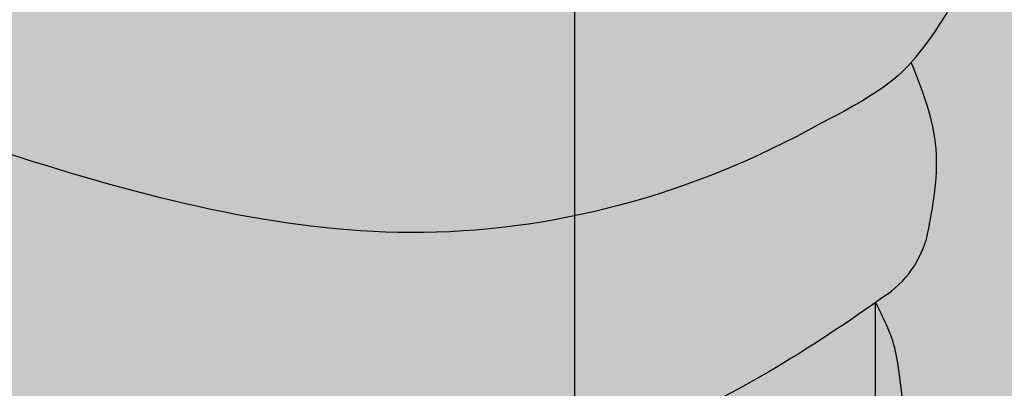
# Model space of a CAD drawing. Units: inches. Extents: x 1704 to 6393, y -157 to 1172.
# Tile 36 of 122: x 2526 to 2564, y 148 to 162. Entities that reach past the tile are written whole.
import ezdxf

# ---------------------------------------------------------------- set-up
doc = ezdxf.new("R2010")
doc.units = ezdxf.units.IN
doc.header["$MEASUREMENT"] = 0
for name, color, linetype, lineweight in [('A-ANNO-DIMS', 7, 'Continuous', 13), ('A-FURN', 8, 'Continuous', 18), ('estofado', 7, 'Continuous', 25)]:
    doc.layers.add(name, color=color, linetype=linetype, lineweight=lineweight)
doc.layers.add('A-FLOR-PATT', color=7, linetype='Continuous', lineweight=13, true_color=0xf2f2f2)
doc.styles.get("Standard").update_dxf_attribs({"font": 'arial.ttf'})
doc.dimstyles.get("Standard").update_dxf_attribs({"dimtxt": 6, "dimasz": 2, "dimexe": 0.18, "dimexo": 0.0625, "dimgap": 0.09, "dimtad": 0, "dimtih": 1, "dimtoh": 1, "dimdec": 1, "dimzin": 0, "dimdsep": 46, "dimlunit": 3, "dimtxsty": 'Standard', "dimblk": 'ARCHTICK', "dimcen": 0.09, "dimadec": 0, "dimazin": 0, "dimtfac": 1, "dimtdec": 1, "dimtofl": 0, "dimtmove": 0, "dimatfit": 3, "dimfxl": 1, "dimtolj": 1, "dimtzin": 0, "dimarcsym": 0})

# ---------------------------------------------------------------- blocks, each defined once
blk = doc.blocks.new('Cama Box Regencia LOLA')
at = {"layer": 'estofado', "ltscale": 0.2}
h = blk.add_hatch(color=256, dxfattribs=at)
h.dxf.hatch_style = 1
h.set_gradient(color1=(240, 232, 219), color2=(213, 190, 154), one_color=1, tint=0.7200000286102295)
edge = h.paths.add_edge_path()
edge.add_line((-0.8000000000000682, -0.1548023628405417), (-0.863597199697665, -0.2293271111754507))
edge.add_spline(control_points=[(-0.8635971996977787, -0.2293271111754507), (-0.8537222782123308, -0.258285373872468), (-0.8269013755602826, -0.3369378214810581), (-0.8674912876567759, -0.4595932758330151), (-0.8253488717912205, -0.6001498518888299), (-0.8771423076391329, -0.7139760714239288), (-0.8243323781925938, -0.8129899320257435), (-0.885044987287756, -0.8716602542656914), (-0.879518062107536, -0.9542863467743244), (-0.8339551707063037, -1.008464155856984), (-0.8245672924600739, -1.059984630119799), (-0.8208601923470268, -1.104655887174089), (-0.8073908324747662, -1.131238421004809), (-0.7999999999999546, -1.145824641594799)], knot_values=[0, 0, 0, 0, 0.0901802310564388, 0.2449351320798513, 0.3646438241986237, 0.5132330690395209, 0.5950634960661151, 0.646820388242338, 0.740988272125753, 0.8098674202588053, 0.8551784313864677, 0.8950360916221496, 0.9434986994854018, 0.9434986994854018, 0.9434986994854018, 0.9434986994854018], degree=3, periodic=0)
edge.add_line((-0.7999999999999546, -1.145824641594856), (-0.7999999999999546, -0.9571831923306604))
edge.add_spline(control_points=[(-0.8000000000001818, -0.9571831923294098), (-0.8003674620557603, -0.9560020588672273), (-0.8014778173377408, -0.9524330433489467), (-0.799534669348418, -0.9460450666617248), (-0.7963405736333016, -0.9382358308520792), (-0.7944188048602429, -0.9289040147384638), (-0.7953122817383474, -0.9190683391483389), (-0.7985341887020923, -0.9137677522519994), (-0.7999999999999546, -0.911356242470788)], knot_values=[0, 0, 0, 0, 0.0036609130031785, 0.0110621328900358, 0.0190316076023675, 0.0292873612819121, 0.0393286152452009, 0.0477100398955968, 0.0477100398955968, 0.0477100398955968, 0.0477100398955968], degree=3, periodic=0)
edge.add_line((-0.8000000000000682, -0.9113562424705037), (-0.7999999999999546, -0.8573491405791173))
edge.add_spline(control_points=[(-0.7999999999999546, -0.8573491405791173), (-0.8011509914009592, -0.8570771933481751), (-0.804102924754261, -0.8563797336621519), (-0.8039036519178353, -0.8498286502876908), (-0.8010279369466388, -0.8413595542568258), (-0.805623441450507, -0.8302818657685406), (-0.801318481758244, -0.8238273834048186), (-0.7999999999999546, -0.8218505664625013)], knot_values=[0, 0, 0, 0, 0.0032305881034183, 0.0082854491905874, 0.015951437769388, 0.0315866871777379, 0.0384893971878813, 0.0384893971878813, 0.0384893971878813, 0.0384893971878813], degree=3, periodic=0)
edge.add_line((-0.7999999999999546, -0.821850566462558), (-0.7999999999999546, -0.7800193173444541))
edge.add_spline(control_points=[(-0.7999999999999546, -0.7800193173443404), (-0.7985416092056994, -0.7788853679199974), (-0.7956241855360986, -0.7766169698310819), (-0.7929439183725436, -0.7707329795046576), (-0.7969680334608711, -0.7644035258254576), (-0.7912681985083055, -0.7566015403456845), (-0.7963938877088595, -0.7483952775559715), (-0.798936373489596, -0.7431699116222604), (-0.799999999999841, -0.7409839258539251)], knot_values=[0, 0, 0, 0, 0.0055481279082489, 0.0110986984731684, 0.0174746050947868, 0.0251556172852474, 0.035519246289823, 0.0429729849735991, 0.0429729849735991, 0.0429729849735991, 0.0429729849735991], degree=3, periodic=0)
edge.add_line((-0.7999999999999546, -0.740983925853584), (-0.8000000000000682, -0.1548023628405417))
h = blk.add_hatch(color=256, dxfattribs=at)
h.dxf.hatch_style = 1
h.set_gradient(color1=(240, 232, 219), color2=(213, 190, 154), one_color=1, tint=0.7200000286102295, name='CURVED')
edge = h.paths.add_edge_path()
edge.add_spline(control_points=[(0.343533776195045, -0.8455058148597345), (0.2879313990920309, -0.8167160606696484), (0.2054770794474052, -0.7744470032542381), (0.0954193394759386, -0.7742416952675626), (-0.0885363502328574, -0.7276964167006668), (0.2428192566063672, -0.7672518992321216), (0.345087521536243, -0.8076697826234067), (0.3825206986321063, -0.8228555492498799)], knot_values=[0.0056315103357428, 0.0056315103357428, 0.0056315103357428, 0.0056315103357428, 0.1860138916206105, 0.2660015162584448, 0.3570871810327863, 0.5963901805690979, 0.739731738908988, 0.739731738908988, 0.739731738908988, 0.739731738908988], degree=3, periodic=0)
edge.add_spline(control_points=[(0.3825206986325611, -0.8228555492497662), (0.3974221570828149, -0.8135511441712424), (0.4121061736600496, -0.8037181558521524), (0.4266849906532571, -0.7937075488799225)], knot_values=[1.358237767273279, 1.358237767273279, 1.358237767273279, 1.358237767273279, 1.409915662372559, 1.409915662372559, 1.409915662372559, 1.409915662372559], degree=3, periodic=0)
edge.add_spline(control_points=[(0.4266849905698109, -0.7937075489369932), (0.3998777739682282, -0.7821381809783361), (0.3476761897024971, -0.7634757898491671), (0.2670618099601825, -0.7565375622627358), (0.0835725072796549, -0.7192994417154637), (0.288524529784695, -0.7446405493717521), (0.4247448861246994, -0.7759943071475277), (0.4449816270193879, -0.7810438091316882)], knot_values=[0.1043639306803623, 0.1043639306803623, 0.1043639306803623, 0.1043639306803623, 0.1896363068641149, 0.2696239315019491, 0.3607095962762907, 0.6000125958126024, 0.6446217338078729, 0.6446217338078729, 0.6446217338078729, 0.6446217338078729], degree=3, periodic=0)
edge.add_spline(control_points=[(0.4449816270197289, -0.7810438091316882), (0.5029779388527232, -0.7406836481117695), (0.5966687145296419, -0.6736247633211292), (0.7071737530245628, -0.6656573253703187), (0.7517012483331201, -0.6672238302253392)], knot_values=[1.43159032281798, 1.43159032281798, 1.43159032281798, 1.43159032281798, 1.63814180148235, 1.770695287284994, 1.770695287284994, 1.770695287284994, 1.770695287284994], degree=3, periodic=0)
edge.add_arc((0.7481853615017826, -0.767162003811734), 0.0999999999999888, 58.7920033978138, 87.98512997550938, ccw=False)
edge.add_line((0.8000000000000682, -0.6816328085782289), (0.8000000000000682, -0.154802362840428))
edge.add_line((0.8000000000000682, -0.154802362840428), (-0.7999999999999546, -0.154802362840428))
edge.add_line((-0.7999999999999546, -0.154802362840428), (-0.8000000000000682, -0.7409839258539819))
edge.add_spline(control_points=[(-0.799999999999841, -0.7409839258539251), (-0.7846451382113174, -0.74846387981205), (-0.7568940913494089, -0.7651582159765554), (-0.7559936909002545, -0.8096905380045313), (-0.7049413305308008, -0.8142555457367848), (-0.7013836936888538, -0.8139988647640733)], knot_values=[0.0122267587020837, 0.0122267587020837, 0.0122267587020837, 0.0122267587020837, 0.0594720782072034, 0.1062176618094138, 0.134458043575382, 0.134458043575382, 0.134458043575382, 0.134458043575382], degree=3, periodic=0)
edge.add_spline(control_points=[(-0.7013836936890812, -0.8139988647637892), (-0.6428309483887916, -0.8132695376718857), (-0.532520673001045, -0.8118955240036598), (-0.2390712668254764, -0.6717984706609172), (-0.3892411364554391, -0.7557901092520752), (-0.4591093260188473, -0.8070101468627512), (-0.5571511178645779, -0.795652750469742), (-0.608497950975675, -0.8409486634728295), (-0.6632498050151981, -0.8266781836207997), (-0.6991149398675134, -0.8254126024436914), (-0.719552182989446, -0.8246914287938125)], knot_values=[0, 0, 0, 0, 0.2187005959148062, 0.4120203559900679, 0.4786136596093368, 0.6046444033330721, 0.6969970394608519, 0.7456449795902803, 0.7925683322559657, 0.8547274388453192, 0.8547274388453192, 0.8547274388453192, 0.8547274388453192], degree=3, periodic=0)
edge.add_spline(control_points=[(-0.7195521829781911, -0.824691428792164), (-0.7293124663336812, -0.8248308281530967), (-0.7545977292818407, -0.8216412233076653), (-0.7742556984202338, -0.794819860189591), (-0.7939222919129634, -0.7820064600295497), (-0.799999999999841, -0.7800193173443404)], knot_values=[0.1564883932805935, 0.1564883932805935, 0.1564883932805935, 0.1564883932805935, 0.184397548386913, 0.2313764834161266, 0.2505984550882281, 0.2505984550882281, 0.2505984550882281, 0.2505984550882281], degree=3, periodic=0)
edge.add_line((-0.8000000000000682, -0.7800193173444541), (-0.7999999999999546, -0.8218505664627286))
edge.add_spline(control_points=[(-0.7999999999999546, -0.8218505664625013), (-0.7938082505512511, -0.8290217081292894), (-0.7673857405620766, -0.8512914803976059), (-0.7619109683460011, -0.8661369353891359), (-0.6555700939965164, -0.8510070218793543), (-0.7139793977868294, -0.8637526923380391), (-0.7379026254519659, -0.8623504601624176), (-0.7688129786438367, -0.8813042143888196), (-0.7854260296310259, -0.8561610219318254), (-0.7961930533253962, -0.8566031243811949), (-0.7999999999999546, -0.8573491405791173)], knot_values=[0.0595743221876141, 0.0595743221876141, 0.0595743221876141, 0.0595743221876141, 0.08075289116965, 0.1037414994169835, 0.1697200936249022, 0.1760361327243865, 0.2071371586311508, 0.2404744334261798, 0.2623408547027293, 0.2736604507987723, 0.2736604507987723, 0.2736604507987723, 0.2736604507987723], degree=3, periodic=0)
edge.add_line((-0.7999999999999546, -0.8573491405791173), (-0.8000000000000682, -0.9113562424721521))
edge.add_spline(control_points=[(-0.8000000000000682, -0.9113562424720385), (-0.7937204054647964, -0.9077594990848183), (-0.7710343135782978, -0.8978798065321029), (-0.7213062468074442, -0.9144666877443228), (-0.6268586829058905, -0.862430497409548), (-0.6896594748232019, -0.9045634991654196), (-0.7483442493064559, -0.9189273406958591), (-0.7835301183422417, -0.922920432793262), (-0.7896301351460125, -0.9477657000142585), (-0.7975786973822779, -0.955260590410262), (-0.8000000000001818, -0.9571831923294098)], knot_values=[0.0138560263374175, 0.0138560263374175, 0.0138560263374175, 0.0138560263374175, 0.0348737775836104, 0.0888666909546002, 0.1078792274429341, 0.1267378491223226, 0.1587140219647659, 0.1937574699451985, 0.2174867851300671, 0.2267221218327879, 0.2267221218327879, 0.2267221218327879, 0.2267221218327879], degree=3, periodic=0)
edge.add_line((-0.7999999999999546, -0.957183192329296), (-0.7999999999999546, -1.145824641594742))
edge.add_spline(control_points=[(-0.8000000000002955, -1.145824641594913), (-0.7271039467997298, -1.094596787649038), (-0.4885706936571524, -0.9465888221489535), (-0.0701640902225336, -0.9707493165000187), (0.237911901821235, -0.902164522332157), (0.3435337762145991, -0.845505814843193)], knot_values=[0.1168958193629841, 0.1168958193629841, 0.1168958193629841, 0.1168958193629841, 0.3797203297758731, 0.9577018633805092, 1.31379338443587, 1.31379338443587, 1.31379338443587, 1.31379338443587], degree=3, periodic=0)
h.paths.add_polyline_path([(-0.6766340706021765, -0.6101327540145576, -0.3575266660906883), (-0.7312746368313583, -0.6354535276154252, -0.3575266660894137), (-0.7059538632299791, -0.5808129613865844, -0.1647847126465284), (-0.7059538632300928, -0.2676124402649407, -0.3575266660890756), (-0.7312746368312446, -0.2129718740360431, -0.3575266660908716), (-0.6766340706020629, -0.2382926476369676, -0.0925607043966334), (-0.1295169377724505, -0.2382926476369107, -0.3575266660898965), (-0.0748763715433825, -0.2129718740360431, -0.3575266660894428), (-0.1001971451446479, -0.2676124402649407, -0.1647847126465285), (-0.1001971451445343, -0.5808129613865844, -0.3575266660890756), (-0.0748763715433825, -0.6354535276154821, -0.3575266660898962), (-0.1295169377724505, -0.6101327540146145, -0.0925607043966531)], flags=16)
h.paths.add_polyline_path([(0.0748763715433825, -0.6354535276157094, -0.3575266660910266), (0.1001971451446479, -0.5808129613865844, -0.1647847126465284), (0.1001971451445343, -0.2676124402649407, -0.3575266660890757), (0.0748763715433825, -0.2129718740360431, -0.3575266660898962), (0.1295169377724505, -0.2382926476369107, -0.0925607043966334), (0.6766340706020629, -0.2382926476369676, -0.3575266660908718), (0.7312746368312446, -0.2129718740360431, -0.3575266660894425), (0.7059538632299791, -0.2676124402649407, -0.1647847126465283), (0.7059538632300928, -0.5808129613865844, -0.3575266660890756), (0.7312746368312446, -0.6354535276154821, -0.3575266660908716), (0.6766340706020629, -0.6101327540145576, -0.0925607043966335), (0.1295169377724505, -0.6101327540146145, -0.3575266660906303)], flags=16)
h = blk.add_hatch(color=256, dxfattribs=at)
h.dxf.hatch_style = 1
h.set_gradient(color1=(206, 178, 131), color2=(227, 212, 186), one_color=1, tint=0.8100000023841857, name='CYLINDER')
edge = h.paths.add_edge_path()
edge.add_arc((0.7481853614966667, -0.7671620038115634), 0.0999999999999888, 342.0511336145294, 447.9851299725766)
edge.add_spline(control_points=[(0.7517012483331201, -0.6672238302253392), (0.7071737530245628, -0.6656573253703187), (0.5966687145298692, -0.6736247633211292), (0.5029779388527232, -0.7406836481117125), (0.4449816270195015, -0.7810438091316314)], knot_values=[1.431590322817835, 1.431590322817835, 1.431590322817835, 1.431590322817835, 1.564143808620479, 1.770695287284994, 1.770695287284994, 1.770695287284994, 1.770695287284994], degree=3, periodic=0)
edge.add_spline(control_points=[(0.4449816270195015, -0.7810438091316314), (0.4388957332065502, -0.7852790380018178), (0.4327996148541616, -0.7895089160493285), (0.4266849906533708, -0.7937075488798087)], knot_values=[1.409915662372814, 1.409915662372814, 1.409915662372814, 1.409915662372814, 1.431590322817835, 1.431590322817835, 1.431590322817835, 1.431590322817835], degree=3, periodic=0)
edge.add_spline(control_points=[(0.4266849906533708, -0.7937075488798087), (0.4121061736600496, -0.8037181558521524), (0.3974221570825875, -0.8135511441712991), (0.38252069863222, -0.8228555492498799)], knot_values=[1.358237767273037, 1.358237767273037, 1.358237767273037, 1.358237767273037, 1.409915662372815, 1.409915662372815, 1.409915662372815, 1.409915662372815], degree=3, periodic=0)
edge.add_line((0.3825206986330158, -0.8228555492493114), (0.343533776286904, -0.8455058148063584))
edge.add_spline(control_points=[(0.3435337761924302, -0.8455058148550165), (0.2379119018048641, -0.902164522335795), (-0.0701640902311738, -0.9707493164995071), (-0.4885706936571524, -0.9465888221488967), (-0.7271039467997298, -1.094596787649038), (-0.8000000000000682, -1.145824641594742)], knot_values=[0.1168958193630798, 0.1168958193630798, 0.1168958193630798, 0.1168958193630798, 0.472987340393773, 1.050968873998409, 1.313793384411202, 1.313793384411202, 1.313793384411202, 1.313793384411202], degree=3, periodic=0)
edge.add_spline(control_points=[(-0.8000000000000682, -1.145824641594742), (-0.8038896190357718, -1.14855807951244), (-0.8077744942224853, -1.151305646504738), (-0.8116551946761774, -1.154065647517199)], knot_values=[0.1028719158199011, 0.1028719158199011, 0.1028719158199011, 0.1028719158199011, 0.1168958193630799, 0.1168958193630799, 0.1168958193630799, 0.1168958193630799], degree=3, periodic=0)
edge.add_arc((-0.7536973518524519, -1.235557294053705), 0.1000000000000352, 125.4208969883762, 169.6981795679068)
edge.add_spline(control_points=[(-0.852085287466366, -1.217673946333093), (-0.8521399740518518, -1.217974812833915), (-0.8565649010855622, -1.242328483616745), (-0.8662697220019026, -1.297321141147904), (-0.8487158298532904, -1.34896742172242), (-0.8348745804664758, -1.381844109035796)], knot_values=[0.3128349436863077, 0.3128349436863077, 0.3128349436863077, 0.3128349436863077, 0.3137509534211996, 0.386958004641742, 0.4759027329026081, 0.4759027329026081, 0.4759027329026081, 0.4759027329026081], degree=3, periodic=0)
edge.add_spline(control_points=[(-0.8348745804664758, -1.38184410903591), (-0.8226532004149476, -1.367823298399059), (-0.8056354908857201, -1.352141651537124), (-0.7460155199962628, -1.32170802000337)], knot_values=[0.0062456970656236, 0.0062456970656236, 0.0062456970656236, 0.0062456970656236, 0.0554759259147193, 0.0554759259147193, 0.0554759259147193, 0.0554759259147193], degree=3, periodic=0)
edge.add_spline(control_points=[(-0.7460155200169539, -1.321708019985464), (-0.6188339616464873, -1.25080943574278), (-0.3488365122128698, -1.179158668568902), (0.0338148848931041, -1.279726484458706), (0.3977250465933366, -1.412092721352792), (0.6449024721503065, -1.106270719748692), (0.7873766543807506, -1.256744909425322), (0.8547271521993025, -1.327877176513538)], knot_values=[0.0991852523588446, 0.0991852523588446, 0.0991852523588446, 0.0991852523588446, 0.5236467270390676, 0.9270872950244264, 1.289918234564769, 1.564439021262726, 1.810554634340498, 1.810554634340498, 1.810554634340498, 1.810554634340498], degree=3, periodic=0)
edge.add_arc((0.5509678495186563, -1.223443291813453), 0.3212104454069235, 341.0267878798241, 383.7782184284114)
edge.add_arc((1.292676354991499, -0.9435407756057543), 0.4723459732861395, 162.0511336103901, 198.5657216587827, ccw=False)
h = blk.add_hatch(color=256, dxfattribs=at)
h.dxf.hatch_style = 1
h.set_gradient(color1=(206, 178, 131), color2=(233, 221, 200), one_color=1, tint=0.8500000238418579, name='CURVED')
edge = h.paths.add_edge_path()
edge.add_spline(control_points=[(0.9233883396182136, -2.254908822900802), (0.9143712174658276, -2.237158585978875), (0.8971704820246486, -2.20329887728792), (0.9295105801843419, -2.140290914518345), (0.848651568119294, -2.10957861148239), (0.9047062348403186, -2.046222426005954), (0.8299480774321636, -1.990932361540615), (0.9387479200587449, -1.92692496801726), (0.8590435458045249, -1.86767849203585), (0.8322262745575699, -1.826028043643361), (0.8247981799574972, -1.810442049687992)], knot_values=[0, 0, 0, 0, 0.0575832900035364, 0.1098437972159638, 0.1698138218664432, 0.2255174829302509, 0.2824861515521905, 0.3632291183773252, 0.4509842065695901, 0.5012091817853866, 0.5012091817853866, 0.5012091817853866, 0.5012091817853866], degree=3, periodic=0)
edge.add_spline(control_points=[(0.8247981799572698, -1.810442049688447), (0.8512430237993839, -1.769990096378137), (0.8869160776755506, -1.705010622333873), (0.9070359522544322, -1.586338752195842), (0.8536462472426364, -1.488247672851343), (0.8944567470317679, -1.387739666353695), (0.8643796102055603, -1.342420998864781), (0.8547271521993025, -1.327877176513538)], knot_values=[0, 0, 0, 0, 0.1438744691785906, 0.2224893870322766, 0.3492927143212738, 0.4561786976395368, 0.5066917301592304, 0.5066917301592304, 0.5066917301592304, 0.5066917301592304], degree=3, periodic=0)
edge.add_spline(control_points=[(0.8547271521993025, -1.327877176513538), (0.7873766543807506, -1.256744909425322), (0.6449024721503065, -1.106270719748692), (0.3977250465933366, -1.412092721352792), (0.0338148848931041, -1.279726484458706), (-0.3488365122128698, -1.179158668568902), (-0.6188339616464873, -1.25080943574278), (-0.7460155200169539, -1.321708019985464)], knot_values=[0.0991852523588446, 0.0991852523588446, 0.0991852523588446, 0.0991852523588446, 0.3453008654366167, 0.6198216521345741, 0.9826525916749167, 1.386093159660275, 1.810554634340498, 1.810554634340498, 1.810554634340498, 1.810554634340498], degree=3, periodic=0)
edge.add_spline(control_points=[(-0.7460155199962628, -1.32170802000337), (-0.8056354908857201, -1.352141651537124), (-0.8226532004149476, -1.367823298399059), (-0.8348745804664758, -1.38184410903591)], knot_values=[0.0062456970656236, 0.0062456970656236, 0.0062456970656236, 0.0062456970656236, 0.0554759259147193, 0.0554759259147193, 0.0554759259147193, 0.0554759259147193], degree=3, periodic=0)
edge.add_spline(control_points=[(-0.8348745804664758, -1.38184410903591), (-0.8364250716851984, -1.383622888820184), (-0.8378983647115774, -1.385374937005849), (-0.8393716577378427, -1.387126985191514)], knot_values=[0, 0, 0, 0, 0.0062456970656236, 0.0062456970656236, 0.0062456970656236, 0.0062456970656236], degree=3, periodic=0)
edge.add_arc((-0.6180450437709624, -1.576392779500167), 0.2912164331649039, 139.4648411061637, 203.3711573294546)
edge.add_arc((-0.7011750866292914, -1.609837078845487), 0.2016528082906132, 204.0179006417974, 212.6189639884946)
edge.add_spline(control_points=[(-0.8710220093900034, -1.718537943240505), (-0.8696870122217887, -1.721658691442996), (-0.8597709916446092, -1.746046247230935), (-0.8464685798230674, -1.804421032451443), (-0.888988689927828, -1.889951451602371), (-0.8378676506146121, -1.973422824210047), (-0.8371590179440318, -2.05992368952792), (-0.8871569320951948, -2.144598622072578), (-0.908935644436724, -2.210906123939594), (-0.9233883398977695, -2.254908823284267)], knot_values=[0, 0, 0, 0, 0.0101500649009363, 0.0785829584511912, 0.1732273504791735, 0.2688802694005398, 0.3498050162211252, 0.4202002266429896, 0.5590752189863636, 0.5590752189863636, 0.5590752189863636, 0.5590752189863636], degree=3, periodic=0)
edge.add_ellipse((-0.9040800600764669, -2.258882422916315), major_axis=(0.0267880171833212, 0.0267880171833213), ratio=0.4535320972039226, start_angle=94.15910660291303, end_angle=123.37101895145429, ccw=False)
edge.add_ellipse((-0.8772920428931456, -2.232094405732993), major_axis=(0.0772920428927364, 0.0772920428927364), ratio=0.168252450050839, start_angle=-1.0527401173021644e-10, end_angle=156.3071135567154, ccw=False)
edge.add_line((-0.8000000000002955, -2.154802362840428), (0.7999592378284888, -2.154802362840428))
edge.add_arc((0.9462065466516378, -2.098298447668867), 0.1567831871334379, 200.9447658774159, 201.1244713640487, ccw=False)
edge.add_arc((1.115979327553759, -2.004946707326951), 0.3497136727815615, 205.2898146244752, 205.3730108333857)
edge.add_ellipse((0.8772920428930319, -2.232094405732993), major_axis=(-0.0772920428927364, 0.0772920428927364), ratio=0.168252450050839, start_angle=203.6928864432847, end_angle=359.99999999994674, ccw=False)
edge.add_ellipse((0.9040800600763532, -2.258882422916315), major_axis=(-0.0267880171833213, 0.0267880171833213), ratio=0.4535320972039226, start_angle=236.6289810485458, end_angle=265.84089339708703, ccw=False)
blk.add_lwpolyline([(-0.7999999999999546, -0.9571831923292393), (-0.7999999999999546, -1.145824641594799)], dxfattribs=at)
for centre, radius, start, end in [((-0.7536973518525656, -1.235557294053876), 0.1, 125.4208969883012, 169.6981794711674), ((-0.618045043771076, -1.576392779500224), 0.2912164331649248, 139.4648411061415, 203.3711573294531)]:
    blk.add_arc(centre, radius, start, end, dxfattribs=at)
for points, knots in [([(-0.8635971996977787, -0.2293271111754507), (-0.8537222782123597, -0.2582853738724713), (-0.8269013755602529, -0.3369378214810687), (-0.8674912876567628, -0.459593275832977), (-0.8253488717912105, -0.6001498518888299), (-0.8771423076387755, -0.7139760714238776), (-0.824332378192706, -0.8129899320257793), (-0.8850449872876955, -0.8716602542656513), (-0.8795180621076731, -0.9542863467744586), (-0.8339551707061605, -1.008464155856879), (-0.8245672924602526, -1.059984630119836), (-0.820860192346876, -1.104655887174075), (-0.8073908324747767, -1.131238421004865), (-0.7999999999999546, -1.145824641594799)], [0, 0, 0, 0, 0.0901802310564388, 0.2449351320798513, 0.3646438241986237, 0.5132330690395209, 0.5950634960661151, 0.646820388242338, 0.740988272125753, 0.8098674202588053, 0.8551784313864677, 0.8950360916221496, 0.9434986994854018, 0.9434986994854018, 0.9434986994854018, 0.9434986994854018]), ([(-0.8116551946761774, -1.154065647517199), (-0.7350455857787211, -1.099579968801037), (-0.493473113061782, -0.9463057365681493), (-0.0701640902311738, -0.9707493164995071), (0.2379119018048641, -0.902164522335795), (0.3435337761924302, -0.8455058148550165)], [0.1028719158199011, 0.1028719158199011, 0.1028719158199011, 0.1028719158199011, 0.3797203297758731, 0.9577018633805092, 1.313793384411202, 1.313793384411202, 1.313793384411202, 1.313793384411202]), ([(-0.7460155200169539, -1.321708019985464), (-0.6188339616464873, -1.25080943574278), (-0.3488365122128698, -1.179158668568902), (0.0338148848931041, -1.279726484458706), (0.3977250465933366, -1.412092721352792), (0.6449024721503065, -1.106270719748692), (0.7873766543807506, -1.256744909425322), (0.8547271521993025, -1.327877176513538)], [0.0991852523588446, 0.0991852523588446, 0.0991852523588446, 0.0991852523588446, 0.5236467270390676, 0.9270872950244264, 1.289918234564769, 1.564439021262726, 1.810554634340498, 1.810554634340498, 1.810554634340498, 1.810554634340498]), ([(-0.852085287466366, -1.217673946333093), (-0.8521399740518518, -1.217974812833915), (-0.8565649010855622, -1.242328483616745), (-0.8662697220019026, -1.297321141147904), (-0.8487158298532904, -1.34896742172242), (-0.8348745804664758, -1.381844109035796)], [0.3128349436863077, 0.3128349436863077, 0.3128349436863077, 0.3128349436863077, 0.3137509534211996, 0.386958004641742, 0.4759027329026081, 0.4759027329026081, 0.4759027329026081, 0.4759027329026081])]:
    blk.add_open_spline(points, degree=3, knots=knots, dxfattribs=at)
for points in [[(-0.8393716577378427, -1.387126985191514), (-0.8262854811396209, -1.371564831868056), (-0.8131993045412855, -1.356002678544541), (-0.7460155199962628, -1.32170802000337)], [(-0.8546555176860692, -1.326056226378227), (-0.8546255600027735, -1.326046411595029), (-0.8545956023194776, -1.326036596811775), (-0.8545656446361817, -1.326026782028861)]]:
    blk.add_open_spline(points, degree=3, dxfattribs=at)
blk = doc.blocks.new('_ArchTick')
at = {"color": 0, "linetype": 'ByBlock', "const_width": 0.15}
blk.add_lwpolyline([(-0.5, -0.5), (0.5, 0.5)], dxfattribs=at)
blk = doc.blocks.new('*D93')
at = {"layer": 'A-ANNO-DIMS', "color": 0, "lineweight": -2, "transparency": 16777216}
for p, q in [((2605.286074000001, 895.2129740000005), (1829.697551000002, 895.2129740000003)), ((1829.877551000002, 895.2129740000003), (1829.877551000002, 495.8664119263302)), ((1829.877551000002, 90.2129739999999), (1829.877551000002, 489.5595360736699)), ((2605.286074000001, 90.21297400000003), (1829.697551000002, 90.2129739999999))]:
    blk.add_line(p, q, dxfattribs=at)
at = {"layer": 'Defpoints', "color": 0, "lineweight": -3, "transparency": 16777216}
for p in [(2605.348574000001, 895.2129740000005), (1829.877551000002, 90.2129739999999), (2605.348574000001, 90.21297400000003)]:
    blk.add_point(p, dxfattribs=at)
at = {"layer": 'A-ANNO-DIMS', "color": 0, "lineweight": -2, "transparency": 16777216, "xscale": 2, "yscale": 2, "zscale": 2}
for p, rotation in [((1829.877551000002, 895.2129740000003), 90), ((1829.877551000002, 90.2129739999999), 270)]:
    blk.add_blockref('_ArchTick', p, dxfattribs=dict(at, rotation=rotation))
at = {"layer": 'A-ANNO-DIMS', "color": 0, "transparency": 16777216, "insert": (1829.877551000001, 492.7129739999994), "char_height": 6, "attachment_point": 5}
blk.add_mtext('\\A1;805', dxfattribs=at)
blk = doc.blocks.new('*D105')
at = {"layer": 'A-ANNO-DIMS', "color": 0, "lineweight": -2, "transparency": 16777216}
for p, q in [((2451.737975, 615.150474), (2451.737975, -64.9670259999999)), ((2547.348574, 615.150474), (2547.348574, -64.9670259999999)), ((2451.737975, -64.787026), (2489.908936164393, -64.787026)), ((2547.348574, -64.787026), (2509.177612835607, -64.787026))]:
    blk.add_line(p, q, dxfattribs=at)
at = {"layer": 'Defpoints', "color": 0, "lineweight": -3, "transparency": 16777216}
for p in [(2451.737975, 615.212974), (2547.348574, 615.212974), (2547.348574, -64.787026)]:
    blk.add_point(p, dxfattribs=at)
at = {"layer": 'A-ANNO-DIMS', "color": 0, "lineweight": -2, "transparency": 16777216, "xscale": 2, "yscale": 2, "zscale": 2, "rotation": 180}
blk.add_blockref('_ArchTick', (2451.737975, -64.787026), dxfattribs=at)
at = {"layer": 'A-ANNO-DIMS', "color": 0, "lineweight": -2, "transparency": 16777216, "xscale": 2, "yscale": 2, "zscale": 2}
blk.add_blockref('_ArchTick', (2547.348574, -64.787026), dxfattribs=at)
at = {"layer": 'A-ANNO-DIMS', "color": 0, "transparency": 16777216, "insert": (2499.5432745, -64.787026), "char_height": 6, "attachment_point": 5}
blk.add_mtext('\\A1;95.61', dxfattribs=at)

msp = doc.modelspace()

# ---------------------------------------------------------------- hatches: boundary and pattern name
at = {"layer": 'A-FLOR-PATT', "transparency": 33554528}
h = msp.add_hatch(color=256, dxfattribs=at)
h.dxf.hatch_style = 1
h.paths.add_polyline_path([(2325.348574056059, 863.2129735309796), (2325.348574056059, 887.2129735309796), (2263.348574056059, 887.2129735309796), (2167.348574056059, 887.2129735309794), (2081.348574056061, 887.2129735309792), (2081.348574056061, 719.2129735309785), (2277.348574056059, 719.2129735309787), (2277.348574056059, 711.2129735309788), (2277.348574056059, 372.212973530979), (2349.348574056059, 372.212973530979), (2381.348574056059, 372.2129735309789), (2381.348574056059, 364.2129735309789), (2353.348574056059, 364.2129735309789), (2353.348574056059, 270.2129735309788), (2381.348574056059, 270.2129735309788), (2381.348574056059, 266.2129735309788), (2357.348574056059, 266.2129735309788), (2357.348574056059, 98.21297353097884), (2381.348574056059, 98.21297353097897), (2385.181056550604, 98.21297353097884), (2386.482186711948, 98.21297353097884), (2424.21496140017, 98.21297353097884), (2425.516091561514, 98.21297353097884), (2429.348574056059, 98.21297353097897), (2597.348574056059, 98.21297353097884), (2597.348574056059, 146.2129735309788), (2597.348574056059, 218.2129735309788), (2597.348574056059, 266.2129735309788), (2423.348574056059, 266.2129735309788), (2423.348574056059, 270.2129735309788), (2473.348574056059, 270.2129735309788), (2473.348574056059, 294.2129735309789), (2477.348574056059, 294.2129735309789), (2477.348574056059, 270.2129735309788), (2547.348574056059, 270.2129735309788), (2547.348574056059, 364.2129735309788), (2477.348574056059, 364.2129735309788), (2477.348574056059, 318.2129735309788), (2473.348574056059, 318.2129735309787), (2473.348574056059, 364.2129735309789), (2423.348574056059, 364.2129735309788), (2423.348574056059, 372.2129735309788), (2469.348574056059, 372.2129735309788), (2469.348574056059, 459.2129735309789), (2469.348574056059, 538.2129735309788), (2350.348574056059, 538.2129735309788), (2350.348574056059, 565.7129735309788), (2358.348574056059, 565.7129735309788), (2358.348574056059, 545.2129735309788), (2420.348574056059, 545.2129735309788), (2420.348574056059, 610.2129735309788), (2358.348574056059, 610.2129735309788), (2358.348574056059, 589.7129735309788), (2350.348574056059, 589.7129735309788), (2350.348574056059, 615.2129735309788), (2425.348574056059, 615.2129735309788), (2425.348574056059, 607.2129735309788), (2425.348574056059, 546.2129735309788), (2469.348574056059, 546.2129735309788), (2514.34857405606, 546.212973530979), (2514.34857405606, 607.2129735309788), (2449.348574056059, 607.2129735309788), (2449.348574056059, 615.2129735309788), (2451.737974987759, 615.2129735309788), (2451.737974987759, 659.2129735309788), (2427.737974987759, 659.2129735309788), (2427.737974987759, 665.2129735309788), (2367.737974987758, 665.2129735309788), (2367.737974987758, 667.2129735309788), (2367.737974987758, 711.2129735309788), (2325.348574056059, 711.2129735309788), (2325.348574056059, 719.2129735309785), (2325.348574056059, 755.2129735309787), (2325.348574056059, 763.2129735309788)])
h.paths.add_polyline_path([(2233.85817000392, 822.532660166629, -0.1872470486944155), (2233.85817000392, 809.1396667958562), (2231.697030374885, 808.8044951349628, 0.0848927708004382), (2233.130501812631, 814.4858417746204), (2230.423974436808, 814.4858417746204, -0.1042581087707907), (2228.553363812687, 808.3129425443484), (2217.750790159711, 807.1555239386723, -0.2222222222222219), (2217.750790159711, 824.5168030238124), (2228.553363812687, 823.3593844181363, -0.1042581087707933), (2230.423974436808, 817.1864851878643), (2233.130501812631, 817.1864851878643, 0.08489277080044), (2231.697030374885, 822.8678318275219)], flags=16)
h.paths.add_polyline_path([(2213.621360876743, 833.1974425663823), (2213.621360876743, 798.4748843961024), (2156.047684459484, 798.4748843961034), (2156.047684459485, 833.1974425663813)], flags=16)
h.paths.add_polyline_path([(2203.931929661768, 848.0987249710489), (2205.089348267444, 837.2961513180724, -0.2222222222222264), (2187.728069182304, 837.2961513180724), (2188.88548778798, 848.0987249710485, -0.104258108770792), (2195.058387018252, 849.9693355951691), (2195.058387018252, 852.6758629709927, 0.084892770800438), (2189.377040378595, 851.2423915332469), (2189.712212039488, 853.4035311622828, -0.1872470486944166), (2203.105205410261, 853.4035311622828), (2203.440377071154, 851.2423915332469, 0.084892770800438), (2197.759030431496, 852.6758629709927), (2197.759030431496, 849.9693355951691, -0.1042581087707896)], flags=16)
h.paths.add_polyline_path([(2181.940976153924, 837.2961513180726, -0.2222222222222323), (2164.579697068783, 837.2961513180724), (2165.73711567446, 848.0987249710487, -0.1042581087707905), (2171.910014904732, 849.9693355951691), (2171.910014904732, 852.6758629709927, 0.0848927708004445), (2166.228668265074, 851.2423915332469), (2166.563839925967, 853.403531162283, -0.1872470486944096), (2179.95683329674, 853.4035311622828), (2180.292004957633, 851.2423915332465, 0.0848927708004458), (2174.610658317976, 852.6758629709927), (2174.610658317976, 849.9693355951691, -0.104258108770801), (2180.783557548248, 848.0987249710482)], flags=16)
h.paths.add_polyline_path([(2205.089348267444, 794.376175644412), (2203.931929661768, 783.5736019914364, -0.1042581087707934), (2197.759030431496, 781.7029913673155), (2197.759030431496, 778.9964639914921, 0.084892770800439), (2203.440377071154, 780.4299354292382), (2203.105205410261, 778.2687958002022, -0.1872470486944172), (2189.712212039488, 778.2687958002018), (2189.377040378595, 780.4299354292377, 0.0848927708004369), (2195.058387018252, 778.9964639914919), (2195.058387018252, 781.7029913673153, -0.1042581087707904), (2188.88548778798, 783.5736019914358), (2187.728069182304, 794.3761756444126, -0.2222222222222231)], flags=16)
h.paths.add_polyline_path([(2181.940976153924, 794.376175644412), (2180.783557548248, 783.5736019914364, -0.1042581087708008), (2174.610658317976, 781.7029913673153), (2174.610658317976, 778.9964639914921, 0.0848927708004458), (2180.292004957633, 780.4299354292382), (2179.95683329674, 778.268795800202, -0.1872470486944096), (2166.563839925967, 778.2687958002018), (2166.228668265074, 780.4299354292378, 0.0848927708004446), (2171.910014904732, 778.9964639914919), (2171.910014904732, 781.7029913673153, -0.1042581087707904), (2165.73711567446, 783.5736019914358), (2164.579697068783, 794.3761756444123, -0.2222222222222294)], flags=16)
h.paths.add_polyline_path([(2151.918255176517, 807.1555239386723), (2141.115681523541, 808.3129425443484, -0.1042581087707911), (2139.24507089942, 814.4858417746204), (2136.538543523597, 814.4858417746204, 0.08489277080044), (2137.972014961343, 808.8044951349626), (2135.810875332307, 809.1396667958562, -0.1872470486944109), (2135.810875332307, 822.5326601666285), (2137.972014961343, 822.8678318275221, 0.0848927708004416), (2136.538543523597, 817.1864851878643), (2139.24507089942, 817.1864851878643, -0.104258108770793), (2141.115681523541, 823.3593844181363), (2151.918255176517, 824.5168030238124, -0.2222222222222205)], flags=16)
h.paths.add_polyline_path([(2357.868011454448, 363.4102250290031), (2358.813881560335, 363.4102250290031, 0.7537604849588476)], flags=16)
h.paths.add_polyline_path([(2372.241054283868, 363.1167008961685), (2372.248110816919, 363.1167008961685), (2372.248110816919, 363.3425764997267), (2371.30224071103, 363.3425764997267), (2371.30224071103, 363.1392706554335, -1.360391292333951)], flags=16)
h.paths.add_polyline_path([(2371.309297244092, 272.7157694655011), (2371.30224071103, 272.7157694655011), (2371.30224071103, 272.4898938619428), (2372.248110816919, 272.4898938619428), (2372.248110816919, 272.6931997062759, -1.360391292393621)], flags=16)
h.paths.add_polyline_path([(2357.875067987504, 272.7157694655011), (2357.868011454452, 272.7157694655011), (2357.868011454452, 272.4898938619428), (2358.813881560341, 272.4898938619428), (2358.813881560341, 272.6931997062361, -1.360391292333948)], flags=16)
h.paths.add_polyline_path([(2353.768696905258, 363.0736921025416), (2376.347425366111, 363.0736921025416), (2376.347425366111, 272.7587782591281), (2353.768696905258, 272.7587782591281)], flags=16)
h.paths.add_polyline_path([(2354.772195947961, 362.0701930598379), (2375.343926323407, 362.0701930598379), (2375.343926323407, 273.7622773018316), (2354.772195947961, 273.7622773018318)], flags=0)
h.paths.add_polyline_path([(2357.868011454452, 363.3425764997267), (2358.813881560341, 363.3425764997266), (2358.813881560341, 363.1167008961684), (2357.868011454452, 363.1167008961684)], flags=16)
h.paths.add_polyline_path([(2359.287941640134, 359.1843485433627), (2359.287941640134, 360.0631949744305), (2370.828180631237, 360.0631949744362), (2370.828180631237, 359.1843485433769), (2374.332057422314, 359.1843485433812), (2374.332057422312, 358.4635369582513), (2372.835178716611, 358.4635369582524), (2372.835178716611, 357.5410357047662), (2374.332057422314, 357.5410357047678), (2374.332057422312, 356.8202241196381), (2372.835178716611, 356.820224119639), (2372.835178716611, 355.897722866153), (2374.332057422314, 355.8977228661546), (2374.332057422312, 355.1769112810248), (2372.835178716611, 355.1769112810259), (2372.835178716611, 354.2544100275397), (2374.332057422334, 354.2544100275415), (2374.332057422331, 353.5335984424117), (2372.835178716631, 353.5335984424126), (2372.835178716631, 352.6110971889265), (2374.332057422334, 352.6110971889282), (2374.332057422331, 351.8902856037984), (2372.835178716631, 351.8902856037993), (2372.835178716631, 350.9677843503132), (2374.332057422334, 350.967784350315), (2374.332057422331, 350.2469727651852), (2372.835178716631, 350.2469727651861), (2372.835178716631, 349.3244715117), (2374.332057422334, 349.3244715117017), (2374.332057422331, 348.603659926572), (2372.835178716631, 348.6036599265729), (2372.835178716631, 347.6811586730868), (2374.332057422334, 347.6811586730886), (2374.332057422331, 346.9603470879587), (2372.835178716631, 346.9603470879598), (2372.835178716631, 346.0378458344735), (2374.332057422334, 346.0378458344753), (2374.332057422331, 345.3170342493456), (2372.835178716631, 345.3170342493465), (2372.835178716631, 344.3945329958605), (2374.332057422334, 344.3945329958621), (2374.332057422331, 343.6737214107324), (2372.835178716631, 343.6737214107334), (2372.835178716631, 342.751220157247), (2374.332057422334, 342.7512201572489), (2374.332057422331, 342.0304085721191), (2372.835178716631, 342.03040857212), (2372.835178716631, 341.1079073186338), (2374.332057422334, 341.1079073186356), (2374.332057422331, 340.3870957335057), (2372.835178716631, 340.3870957335066), (2372.835178716631, 339.4645944800207), (2374.332057422334, 339.4645944800223), (2374.332057422331, 338.7437828948924), (2372.835178716648, 338.7437828948933), (2372.835178716648, 337.8212816414076), (2374.332057422334, 337.8212816414093), (2374.332057422331, 337.1004700562794), (2372.835178716648, 337.1004700562803), (2372.835178716648, 336.1779688027942), (2374.332057422334, 336.1779688027961), (2374.332057422331, 335.4571572176662), (2372.835178716648, 335.4571572176673), (2372.835178716648, 334.5346559641809), (2374.332057422334, 334.5346559641828), (2374.332057422331, 333.8138443790529), (2372.835178716648, 333.8138443790539), (2372.835178716648, 332.8913431255679), (2374.332057422334, 332.8913431255696), (2374.332057422331, 332.1705315404397), (2372.835178716648, 332.1705315404406), (2372.835178716648, 331.2480302869545), (2374.332057422334, 331.2480302869563), (2374.332057422331, 330.5272187018265), (2372.835178716648, 330.5272187018273), (2372.835178716648, 329.6047174483413), (2374.332057422334, 329.6047174483431), (2374.332057422331, 328.8839058632133), (2372.835178716648, 328.8839058632143), (2372.835178716648, 327.9614046097282), (2374.332057422334, 327.9614046097298), (2374.332057422331, 327.2405930246), (2372.835178716648, 327.2405930246009), (2372.835178716648, 326.3180917711149), (2374.332057422334, 326.3180917711167), (2374.332057422331, 325.5972801859869), (2372.835178716648, 325.5972801859877), (2372.835178716648, 324.6747789325016), (2374.332057422334, 324.6747789325034), (2374.332057422331, 323.9539673473736), (2372.835178716648, 323.9539673473746), (2372.835178716648, 323.0314660938884), (2374.332057422334, 323.0314660938901), (2374.332057422331, 322.3106545087603), (2372.835178716648, 322.3106545087613), (2372.835178716648, 321.3881532552753), (2374.332057422334, 321.388153255277), (2374.332057422331, 320.6673416701471), (2372.835178716648, 320.6673416701481), (2372.835178716648, 319.7448404166621), (2374.332057422334, 319.7448404166638), (2374.332057422331, 319.0240288315339), (2372.835178716648, 319.0240288315348), (2372.835178716648, 318.1015275780487), (2374.332057422334, 318.1015275780504), (2374.332057422331, 317.3807159929205), (2372.835178716648, 317.3807159929214), (2372.835178716648, 316.4582147394357), (2374.332057422334, 316.4582147394373), (2374.332057422331, 315.7374031543073), (2372.835178716648, 315.7374031543084), (2372.835178716648, 314.8149019008223), (2374.332057422334, 314.8149019008241), (2374.332057422331, 314.0940903156943), (2372.835178716648, 314.0940903156952), (2372.835178716648, 313.171589062209), (2374.332057422334, 313.1715890622108), (2374.332057422331, 312.450777477081), (2372.835178716648, 312.4507774770819), (2372.835178716648, 311.5282762235959), (2374.332057422334, 311.5282762235977), (2374.332057422331, 310.8074646384678), (2372.835178716648, 310.8074646384687), (2372.835178716648, 309.8849633849827), (2374.332057422334, 309.8849633849844), (2374.332057422331, 309.1641517998546), (2372.835178716648, 309.1641517998555), (2372.835178716648, 308.2416505463693), (2374.332057422334, 308.2416505463712), (2374.332057422331, 307.5208389612412), (2372.835178716648, 307.5208389612421), (2372.835178716648, 306.5983377077562), (2374.332057422334, 306.598337707758), (2374.332057422331, 305.8775261226281), (2372.835178716648, 305.8775261226289), (2372.835178716648, 304.955024869143), (2374.332057422334, 304.9550248691447), (2374.332057422331, 304.2342132840149), (2372.835178716648, 304.2342132840158), (2372.835178716648, 303.3117120305298), (2374.332057422334, 303.3117120305316), (2374.332057422331, 302.5909004454018), (2372.835178716648, 302.5909004454027), (2372.835178716648, 301.6683991919165), (2374.332057422334, 301.6683991919183), (2374.332057422331, 300.9475876067885), (2372.835178716648, 300.9475876067894), (2372.835178716648, 300.0250863533033), (2374.332057422334, 300.025086353305), (2374.332057422331, 299.3042747681752), (2372.835178716648, 299.3042747681761), (2372.835178716648, 298.3817735146902), (2374.332057422334, 298.3817735146919), (2374.332057422331, 297.6609619295621), (2372.835178716648, 297.6609619295629), (2372.835178716648, 296.7384606760769), (2374.332057422334, 296.7384606760786), (2374.332057422331, 296.0176490909488), (2372.835178716648, 296.0176490909498), (2372.835178716648, 295.0951478374636), (2374.332057422334, 295.0951478374653), (2374.332057422331, 294.3743362523355), (2372.835178716648, 294.3743362523364), (2372.835178716648, 293.4518349988504), (2374.332057422334, 293.4518349988522), (2374.332057422331, 292.7310234137224), (2372.835178716648, 292.7310234137233), (2372.835178716648, 291.8085221602371), (2374.332057422334, 291.8085221602389), (2374.332057422331, 291.0877105751091), (2372.835178716648, 291.08771057511), (2372.835178716648, 290.165209321624), (2374.332057422334, 290.1652093216256), (2374.332057422331, 289.4443977364957), (2372.835178716648, 289.4443977364966), (2372.835178716648, 288.5218964830108), (2374.332057422334, 288.5218964830125), (2374.332057422331, 287.8010848978827), (2372.835178716648, 287.8010848978836), (2372.835178716648, 286.8785836443975), (2374.332057422334, 286.8785836443993), (2374.332057422331, 286.1577720592695), (2372.835178716648, 286.1577720592703), (2372.835178716648, 285.2352708057842), (2374.332057422334, 285.2352708057861), (2374.332057422331, 284.5144592206562), (2372.835178716648, 284.514459220657), (2372.835178716648, 283.5919579671712), (2374.332057422334, 283.5919579671728), (2374.332057422331, 282.871146382043), (2372.835178716648, 282.8711463820439), (2372.835178716648, 281.9486451285579), (2374.332057422334, 281.9486451285596), (2374.332057422331, 281.2278335434298), (2372.835178716648, 281.2278335434307), (2372.835178716648, 280.3053322899446), (2374.332057422334, 280.3053322899464), (2374.332057422331, 279.5845207048164), (2372.835178716648, 279.5845207048174), (2372.835178716648, 278.6620194513314), (2374.332057422334, 278.6620194513331), (2374.332057422331, 277.9412078662033), (2372.835178716648, 277.9412078662043), (2372.835178716648, 277.0187066127184), (2374.332057422334, 277.0187066127201), (2374.332057422331, 276.29789502759), (2370.828180631244, 276.2978950275922), (2370.828180631244, 275.7692753872335), (2359.287941640128, 275.7692753872392), (2359.287941640128, 276.2978950275993), (2355.784064849037, 276.2978950276015), (2355.784064849037, 277.0187066126971), (2357.280943554723, 277.0187066126989), (2357.280943554723, 277.9412078662137), (2355.784064849037, 277.9412078662145), (2355.784064849037, 278.6620194513103), (2357.280943554723, 278.6620194513122), (2357.280943554723, 279.5845207048271), (2355.784064849037, 279.584520704828), (2355.784064849037, 280.3053322899236), (2357.280943554723, 280.3053322899253), (2357.280943554723, 281.2278335434403), (2355.784064849037, 281.2278335434412), (2355.784064849037, 281.9486451285369), (2357.280943554723, 281.9486451285387), (2357.280943554723, 282.8711463820535), (2355.784064849037, 282.8711463820543), (2355.784064849037, 283.5919579671501), (2357.280943554723, 283.591957967152), (2357.280943554723, 284.5144592206668), (2355.784064849037, 284.5144592206676), (2355.784064849037, 285.2352708057632), (2357.280943554723, 285.2352708057651), (2357.280943554723, 286.1577720592801), (2355.784064849037, 286.1577720592809), (2355.784064849037, 286.8785836443766), (2357.280943554723, 286.8785836443784), (2357.280943554723, 287.8010848978931), (2355.784064849037, 287.8010848978941), (2355.784064849037, 288.5218964829895), (2357.280943554723, 288.5218964829913), (2357.280943554723, 289.4443977365064), (2355.784064849037, 289.4443977365072), (2355.784064849037, 290.1652093216029), (2357.280943554723, 290.1652093216047), (2357.280943554723, 291.0877105751197), (2355.784064849037, 291.0877105751206), (2355.784064849037, 291.8085221602161), (2357.280943554723, 291.8085221602179), (2357.280943554723, 292.7310234137328), (2355.784064849037, 292.7310234137337), (2355.784064849037, 293.4518349988293), (2357.280943554723, 293.451834998831), (2357.280943554723, 294.3743362523461), (2355.784064849037, 294.3743362523469), (2355.784064849037, 295.0951478374426), (2357.280943554723, 295.0951478374445), (2357.280943554723, 296.0176490909594), (2355.784064849037, 296.0176490909601), (2355.784064849037, 296.7384606760557), (2357.280943554723, 296.7384606760575), (2357.280943554723, 297.6609619295724), (2355.784064849037, 297.6609619295734), (2355.784064849037, 298.3817735146691), (2357.280943554723, 298.3817735146709), (2357.280943554723, 299.3042747681858), (2355.784064849037, 299.3042747681866), (2355.784064849037, 300.0250863532823), (2357.280943554723, 300.0250863532841), (2357.280943554723, 300.9475876067989), (2355.784064849037, 300.9475876067997), (2355.784064849037, 301.6683991918954), (2357.280943554723, 301.6683991918973), (2357.280943554723, 302.5909004454123), (2355.784064849037, 302.5909004454133), (2355.784064849037, 303.3117120305088), (2357.280943554723, 303.3117120305105), (2357.280943554723, 304.2342132840254), (2355.784064849037, 304.2342132840262), (2355.784064849037, 304.9550248691219), (2357.280943554723, 304.9550248691238), (2357.280943554723, 305.8775261226386), (2355.784064849037, 305.8775261226394), (2355.784064849037, 306.5983377077352), (2357.280943554723, 306.5983377077369), (2357.280943554723, 307.5208389612518), (2355.784064849037, 307.5208389612528), (2355.784064849037, 308.2416505463484), (2357.280943554723, 308.2416505463501), (2357.280943554723, 309.1641517998652), (2355.784064849037, 309.1641517998661), (2355.784064849037, 309.8849633849617), (2357.280943554723, 309.8849633849634), (2357.280943554723, 310.8074646384782), (2355.784064849037, 310.8074646384791), (2355.784064849037, 311.5282762235748), (2357.280943554723, 311.5282762235767), (2357.280943554723, 312.4507774770916), (2355.784064849037, 312.4507774770925), (2355.784064849037, 313.171589062188), (2357.280943554723, 313.1715890621898), (2357.280943554723, 314.0940903157049), (2355.784064849037, 314.0940903157058), (2355.784064849037, 314.8149019008013), (2357.280943554723, 314.8149019008032), (2357.280943554723, 315.7374031543179), (2355.784064849037, 315.7374031543187), (2355.784064849037, 316.4582147394146), (2357.280943554723, 316.4582147394165), (2357.280943554723, 317.3807159929311), (2355.784064849037, 317.3807159929321), (2355.784064849037, 318.1015275780277), (2357.280943554723, 318.1015275780295), (2357.280943554723, 319.0240288315445), (2355.784064849037, 319.0240288315454), (2355.784064849037, 319.744840416641), (2357.280943554723, 319.7448404166428), (2357.280943554723, 320.6673416701576), (2355.784064849037, 320.6673416701585), (2355.784064849037, 321.3881532552541), (2357.280943554723, 321.388153255256), (2357.280943554723, 322.3106545087708), (2355.784064849037, 322.3106545087718), (2355.784064849037, 323.0314660938674), (2357.280943554723, 323.0314660938692), (2357.280943554723, 323.9539673473843), (2355.784064849037, 323.9539673473851), (2355.784064849037, 324.6747789324806), (2357.280943554723, 324.6747789324824), (2357.280943554723, 325.5972801859974), (2355.784064849037, 325.5972801859983), (2355.784064849037, 326.3180917710939), (2357.280943554723, 326.3180917710958), (2357.280943554723, 327.2405930246105), (2355.784064849037, 327.2405930246113), (2355.784064849037, 327.9614046097071), (2357.280943554723, 327.961404609709), (2357.280943554723, 328.8839058632238), (2355.784064849037, 328.8839058632245), (2355.784064849037, 329.6047174483202), (2357.280943554723, 329.604717448322), (2357.280943554723, 330.527218701837), (2355.784064849037, 330.5272187018379), (2355.784064849037, 331.2480302869335), (2357.280943554723, 331.2480302869353), (2357.280943554723, 332.1705315404502), (2355.784064849037, 332.170531540451), (2355.784064849037, 332.8913431255468), (2357.280943554723, 332.8913431255486), (2357.280943554723, 333.8138443790634), (2355.784064849037, 333.8138443790642), (2355.784064849037, 334.5346559641599), (2357.280943554723, 334.5346559641618), (2357.280943554723, 335.4571572176767), (2355.784064849037, 335.4571572176776), (2355.784064849037, 336.1779688027732), (2357.280943554723, 336.177968802775), (2357.280943554723, 337.1004700562898), (2355.784064849037, 337.1004700562908), (2355.784064849037, 337.8212816413864), (2357.280943554723, 337.8212816413883), (2357.280943554723, 338.7437828949031), (2355.784064849037, 338.743782894904), (2355.784064849037, 339.4645944799996), (2357.280943554706, 339.4645944800013), (2357.280943554706, 340.3870957335163), (2355.784064849037, 340.3870957335173), (2355.784064849037, 341.1079073186129), (2357.280943554706, 341.1079073186146), (2357.280943554706, 342.0304085721296), (2355.784064849037, 342.0304085721304), (2355.784064849037, 342.7512201572262), (2357.280943554706, 342.751220157228), (2357.280943554706, 343.6737214107429), (2355.784064849037, 343.6737214107437), (2355.784064849037, 344.3945329958394), (2357.280943554706, 344.3945329958412), (2357.280943554706, 345.317034249356), (2355.784064849037, 345.3170342493569), (2355.784064849037, 346.0378458344526), (2357.280943554706, 346.0378458344544), (2357.280943554706, 346.9603470879692), (2355.784064849037, 346.9603470879701), (2355.784064849037, 347.6811586730658), (2357.280943554706, 347.6811586730677), (2357.280943554706, 348.6036599265824), (2355.784064849037, 348.6036599265833), (2355.784064849037, 349.324471511679), (2357.280943554706, 349.3244715116809), (2357.280943554706, 350.2469727651956), (2355.784064849037, 350.2469727651966), (2355.784064849037, 350.9677843502922), (2357.280943554706, 350.9677843502939), (2357.280943554706, 351.8902856038089), (2355.784064849037, 351.8902856038098), (2355.784064849037, 352.6110971889055), (2357.280943554706, 352.6110971889072), (2357.280943554706, 353.5335984424222), (2355.784064849037, 353.533598442423), (2355.784064849037, 354.2544100275187), (2357.280943554686, 354.2544100275204), (2357.280943554686, 355.1769112810354), (2355.784064849017, 355.1769112810362), (2355.784064849017, 355.897722866132), (2357.280943554686, 355.8977228661338), (2357.280943554686, 356.8202241196486), (2355.784064849017, 356.8202241196495), (2355.784064849017, 357.5410357047453), (2357.280943554686, 357.5410357047471), (2357.280943554686, 358.4635369582618), (2355.784064849017, 358.4635369582626), (2355.784064849017, 359.1843485433584)], flags=0)

# ---------------------------------------------------------------- block references
at = {"layer": 'A-FURN', "xscale": 39.22313671019584, "yscale": 39.22313671019584, "zscale": 39.22313671019584, "rotation": 180}
msp.add_blockref('Cama Box Regencia LOLA', (2527.569415053021, 106.0625493409584), dxfattribs=at)

# ---------------------------------------------------------------- dimensions: what is measured, and where the dimension line sits
at = {"layer": 'A-ANNO-DIMS'}
dim = msp.add_linear_dim(base=(1829.877551000002, 90.2129739999999), p1=(2605.348574000001, 895.212974), p2=(2605.348574000001, 90.21297399999999), angle=90, dimstyle='Standard', override={"dimdec": 0, "dimlfac": 1, "dimrnd": 0, "dimzin": 0, "dimdsep": 46, "dimlunit": 2}, dxfattribs=at)
dim.commit()
dim.dimension.update_dxf_attribs({"geometry": '*D93', "text_midpoint": (1829.877551000001, 492.7129739999994)})
dim = msp.add_linear_dim(base=(2547.348574, -64.787026), p1=(2451.737975, 615.212974), p2=(2547.348574, 615.212974), dimstyle='Standard', override={"dimdec": 2, "dimlfac": 1, "dimrnd": 0, "dimzin": 0, "dimdsep": 46, "dimlunit": 2}, dxfattribs=at)
dim.commit()
dim.dimension.update_dxf_attribs({"geometry": '*D105', "text_midpoint": (2499.5432745, -64.787026)})

doc.saveas('drawing.dxf')
